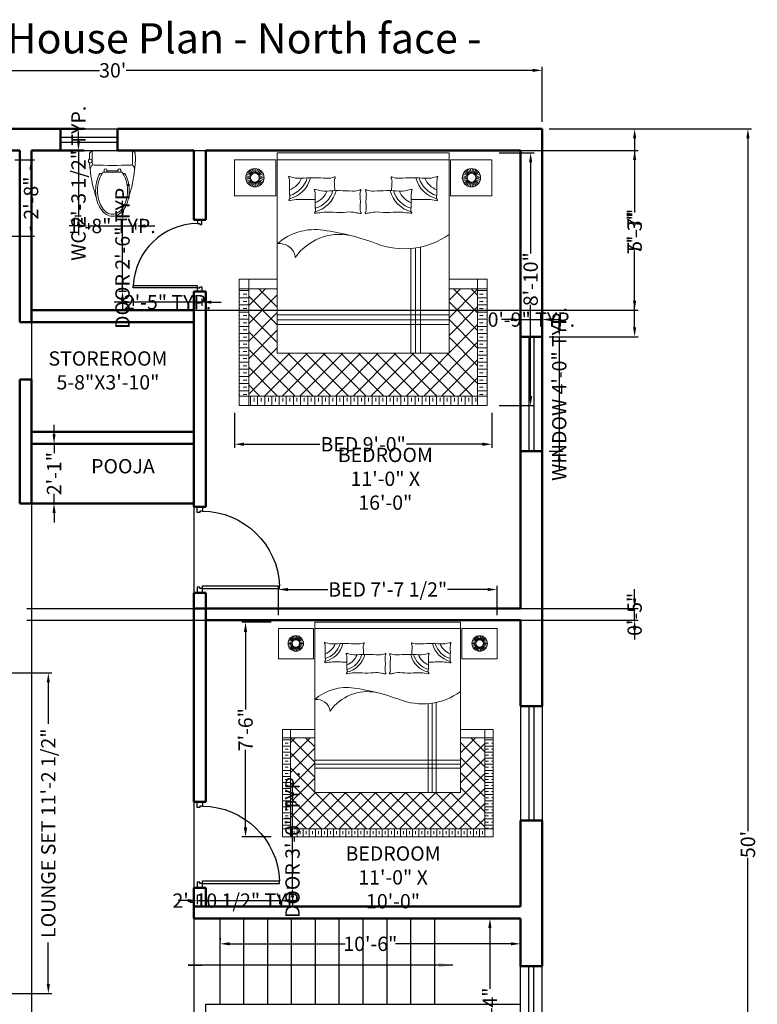
# Model space of a CAD drawing. Units: inches. Extents: x 234 to 707, y 260 to 1025.
# Tile 3 of 3: x 398 to 707, y 612 to 1025. Entities that reach past the tile are written whole.
import ezdxf

# ---------------------------------------------------------------- set-up
doc = ezdxf.new("R2010")
doc.units = ezdxf.units.IN
doc.header["$MEASUREMENT"] = 0
for name, color, linetype, lineweight in [('A-ANNO-DIMS', 3, 'Continuous', 18), ('A-ANNO-SYMB', 3, 'Continuous', 18), ('A-ANNO-TEXT', 7, 'Continuous', 35), ('A-AREA-IDEN', 7, 'Continuous', 25), ('A-DOOR', 2, 'Continuous', 25), ('A-FLOR-CASE', 30, 'Continuous', 25), ('A-FLOR-FIXT', 9, 'Continuous', 18), ('A-FLOR-STRS', 4, 'Continuous', 25), ('A-FURN', 9, 'Continuous', 18), ('WALL', 7, 'Continuous', 50), ('WINDOW', 2, 'Continuous', 25)]:
    doc.layers.add(name, color=color, linetype=linetype, lineweight=lineweight)
doc.styles.get("Standard").update_dxf_attribs({"font": 'arial.ttf'})
doc.styles.add('YQ_DIM', font='SUPEROS.SHX', dxfattribs={"width": 0.8, "bigfont": 'HZDX.SHX'})
doc.dimstyles.new('yqi0', dxfattribs={"dimscale": 0, "dimtxt": 6, "dimasz": 4, "dimexe": 1.5, "dimexo": 3, "dimgap": 0.5, "dimtad": 0, "dimdec": 1, "dimdsep": 46, "dimlunit": 4, "dimtxsty": 'Standard', "dimcen": 0, "dimclrd": 256, "dimclre": 256, "dimclrt": 7, "dimadec": 1, "dimazin": 2, "dimtfac": 1, "dimtdec": 1, "dimtix": 1, "dimtmove": 2, "dimatfit": 2, "dimfxl": 1, "dimtolj": 1, "dimtzin": 0, "dimarcsym": 0})

# ---------------------------------------------------------------- blocks, each defined once
blk = doc.blocks.new('*D2')
at = {"layer": 'A-ANNO-DIMS', "color": 0, "lineweight": -2, "transparency": 16777216}
for p, q in [((257.21, 981.74), (257.21, 1004.79)), ((261.21, 1003.29), (431.62, 1003.29)), ((613.21, 1003.29), (442.8, 1003.29)), ((617.21, 981.74), (617.21, 1004.79))]:
    blk.add_line(p, q, dxfattribs=at)
at = {"layer": 'A-ANNO-DIMS', "color": 0, "transparency": 16777216}
for points in [[(261.21, 1003.95), (261.21, 1002.62), (257.21, 1003.29)], [(613.21, 1003.95), (613.21, 1002.62), (617.21, 1003.29)]]:
    blk.add_solid(points, dxfattribs=at)
at = {"layer": 'Defpoints', "color": 0, "transparency": 16777216}
for p in [(617.21, 1003.29), (257.21, 978.74), (617.21, 978.74)]:
    blk.add_point(p, dxfattribs=at)
at = {"layer": 'A-ANNO-DIMS', "color": 0, "transparency": 16777216, "insert": (437.21, 1003.29), "char_height": 6, "attachment_point": 5}
blk.add_mtext("\\A1;30'", dxfattribs=at)
blk = doc.blocks.new('*D3')
at = {"layer": 'A-ANNO-DIMS', "color": 0, "lineweight": -2, "transparency": 16777216}
for p, q in [((620.21, 978.74), (705.01, 978.74)), ((703.51, 974.74), (703.51, 684.33)), ((703.51, 382.74), (703.51, 673.15)), ((620.21, 378.74), (705.01, 378.74))]:
    blk.add_line(p, q, dxfattribs=at)
at = {"layer": 'A-ANNO-DIMS', "color": 0, "transparency": 16777216}
for points in [[(702.84, 974.74), (704.17, 974.74), (703.51, 978.74)], [(702.84, 382.74), (704.17, 382.74), (703.51, 378.74)]]:
    blk.add_solid(points, dxfattribs=at)
at = {"layer": 'Defpoints', "color": 0, "transparency": 16777216}
for p in [(617.21, 978.74), (617.21, 378.74), (703.51, 378.74)]:
    blk.add_point(p, dxfattribs=at)
at = {"layer": 'A-ANNO-DIMS', "color": 0, "transparency": 16777216, "insert": (703.51, 678.74), "char_height": 6, "attachment_point": 5, "rotation": 90}
blk.add_mtext("\\A1;50'", dxfattribs=at)
blk = doc.blocks.new('DR_D01')
for p, q in [((-0.45, 0.93), (-0.42, 0.93)), ((-0.45, 0.03), (-0.45, 0.93)), ((-0.42, 0.03), (-0.42, 0.93)), ((-0.5, 0.03), (-0.42, 0.03)), ((-0.5, 0.03), (-0.5, -0.03)), ((-0.45, 0.03), (-0.45, 0)), ((-0.45, 0), (-0.435, 0)), ((-0.435, 0), (-0.435, -0.03)), ((0.435, 0), (0.435, -0.03)), ((0.45, 0), (0.435, 0)), ((0.45, 0.03), (0.45, 0)), ((0.5, 0.03), (0.45, 0.03)), ((0.5, -0.03), (0.5, 0.03)), ((-0.435, -0.03), (-0.5, -0.03)), ((0.435, -0.03), (0.5, -0.03))]:
    blk.add_line(p, q)
blk.add_arc((-0.46, 0.021), 0.91, 0.5915, 87.4664)
blk = doc.blocks.new('WD_WIN4')
for p, q in [((-0.5, 0.5), (0.5, 0.5)), ((-0.5, 0.12), (0.5, 0.12)), ((-0.5, -0.12), (0.5, -0.12)), ((-0.5, -0.5), (0.5, -0.5))]:
    blk.add_line(p, q)
blk = doc.blocks.new('yq_matong_01')
for p, q in [((20, 221), (139, 221)), ((0, 201), (0, -201)), ((252, 138), (252, 114)), ((216, 91), (238, 91)), ((216, 61), (238, 61)), ((223, 61), (223, -61)), ((238, 104), (238, -104)), ((216, -61), (238, -61)), ((216, -91), (238, -91)), ((252, -114), (252, -138)), ((20, -221), (139, -221)), ((97, -221), (97, -226)), ((97, -226), (132, -226)), ((132, -221), (132, -226))]:
    blk.add_line(p, q)
for centre, radius, start, end in [((55, 202), 54.8, 117.322, 181.8992), ((20, 201), 20, 90, 180), ((64, -1165), 1417, 71.4068, 91.3856), ((139, 201), 20, 2.3063, 90), ((217, 161), 83.2, 95.4963, 139.9324), ((-4840, 0), 5003, 357.6937, 2.3063), ((357, -47), 193, 123.2779, 128.1384), ((407, -123), 283, 105.2088, 123.2779), ((407, -123), 303, 105.2088, 120.5699), ((439, -242), 427, 74.7912, 105.2088), ((439, -242), 407, 74.7912, 105.2088), ((471, -123), 283, 56.7221, 74.7912), ((471, -123), 303, 56.7221, 74.7912), ((521, -47), 193, 32.2565, 56.7221), ((521, -47), 213, 32.2565, 56.7221), ((216, 76), 15, 90, 270), ((596, 0), 104, 360, 32.2565), ((596, 0), 124, 360, 32.2565), ((216, -76), 15, 90, 270), ((357, 47), 193, 231.8616, 236.7221), ((521, 47), 193, 303.2779, 327.7435), ((521, 47), 213, 303.2779, 327.7435), ((596, 0), 104, 327.7435, 360), ((596, 0), 124, 327.7435, 360), ((51, -204), 51.4, 175.687, 245.0918), ((20, -201), 20, 180, 270), ((64, 1165), 1417, 272.8967, 288.5932), ((139, -201), 20, 270, 357.6937), ((217, -161), 83.2, 220.0676, 264.5037), ((407, 123), 283, 236.7221, 254.7912), ((407, 123), 303, 239.4301, 254.7912), ((439, 242), 427, 254.7912, 285.2088), ((439, 242), 407, 254.7912, 285.2088), ((471, 123), 283, 285.2088, 303.2779), ((471, 123), 303, 285.2088, 303.2779), ((64, 1165), 1417, 268.6144, 271.2036), ((157, -247), 63.1, 159.6834, 188.4939), ((114, -226), 37, 237.5287, 304.2772), ((72, -247), 63.1, 352.0944, 20.3166)]:
    blk.add_arc(centre, radius, start, end)
blk = doc.blocks.new('BED')
h = blk.add_hatch()
h.set_pattern_fill('TRANS', color=256, scale=12, style=0)
h.set_pattern_definition([(360, (4433.967, -9715.0492), (1e-15, 3), []), (360, (4433.967, -9713.5492), (1e-15, 3), [1.5, -1.5])])
h.paths.add_polyline_path([(48, -103), (52, -103), (52, -58), (48, -58)])
h.paths.add_polyline_path([(-48, -58), (-52, -58), (-52, -103), (-48, -103)])
h = blk.add_hatch()
h.set_pattern_fill('ANSI37', color=256, scale=42, angle=-90, style=0)
h.set_pattern_definition([(315, (7787.1367, 4477.8466), (3.7123106, 3.7123106), []), (45, (7787.1367, 4477.8466), (-3.7123106, 3.7123106), [])])
h.paths.add_polyline_path([(-36, -85), (-36, -58), (-48, -58), (-48, -103), (48, -103), (48, -58), (36, -58), (36, -85)])
h = blk.add_hatch()
h.set_pattern_fill('TRANS', color=256, scale=12, angle=-90, style=0)
h.set_pattern_definition([(270, (4433.967, -9715.0492), (3, -1e-15), []), (270, (4435.467, -9715.0492), (3, -1e-15), [1.5, -1.5])])
h.paths.add_polyline_path([(48, -107), (48, -103), (-48, -103), (-48, -107)])
for p, q in [((-54, -4), (-54, -19)), ((-36.64, -4), (-54, -4)), ((-36.64, -4), (-36.64, -19)), ((-36, -1), (36, -1)), ((-36, -85), (-36, -1)), ((-36, -4), (36, -4)), ((36, -1), (36, -85)), ((36.64, -4), (36.64, -19)), ((36.64, -4), (54, -4)), ((54, -4), (54, -19)), ((-46.31, -9.86), (-47.31, -8.13)), ((-45.96, -9.7), (-46.58, -7.8)), ((-45.58, -9.62), (-45.8, -7.63)), ((-45.2, -9.62), (-45, -7.63)), ((-44.82, -9.7), (-44.21, -7.79)), ((-44.47, -9.85), (-43.48, -8.12)), ((44.47, -9.85), (43.48, -8.12)), ((44.82, -9.7), (44.21, -7.79)), ((45.2, -9.62), (45, -7.63)), ((45.58, -9.62), (45.8, -7.63)), ((45.96, -9.7), (46.58, -7.8)), ((46.31, -9.86), (47.31, -8.13)), ((-47.23, -11.45), (-49.23, -11.45)), ((-47.19, -11.07), (-49.14, -10.66)), ((-47.19, -11.83), (-49.14, -12.25)), ((-47.07, -10.7), (-48.9, -9.89)), ((-47.07, -12.2), (-48.89, -13.01)), ((-46.88, -10.37), (-48.5, -9.2)), ((-46.62, -10.08), (-47.96, -8.6)), ((-44.16, -10.08), (-42.83, -8.59)), ((-43.9, -10.36), (-42.29, -9.18)), ((-43.71, -10.7), (-41.89, -9.88)), ((-43.71, -12.19), (-41.88, -13)), ((-43.59, -11.06), (-41.64, -10.64)), ((-43.59, -11.83), (-41.63, -12.24)), ((-43.55, -11.44), (-41.55, -11.44)), ((43.55, -11.44), (41.55, -11.44)), ((43.59, -11.83), (41.63, -12.24)), ((43.59, -11.06), (41.64, -10.64)), ((43.71, -12.19), (41.88, -13)), ((43.71, -10.7), (41.89, -9.88)), ((43.9, -10.36), (42.29, -9.18)), ((44.16, -10.08), (42.83, -8.59)), ((46.62, -10.08), (47.96, -8.6)), ((46.88, -10.37), (48.5, -9.2)), ((47.07, -10.7), (48.9, -9.89)), ((47.07, -12.2), (48.89, -13.01)), ((47.19, -11.07), (49.14, -10.66)), ((47.19, -11.83), (49.14, -12.25)), ((47.23, -11.45), (49.23, -11.45)), ((-46.87, -12.53), (-48.49, -13.71)), ((-46.62, -12.81), (-47.95, -14.3)), ((-46.3, -13.04), (-47.3, -14.77)), ((-45.95, -13.2), (-46.57, -15.1)), ((-45.58, -13.27), (-45.78, -15.26)), ((-45.19, -13.27), (-44.98, -15.26)), ((-44.82, -13.19), (-44.2, -15.09)), ((-44.47, -13.04), (-43.46, -14.77)), ((-44.16, -12.81), (-42.82, -14.29)), ((-43.9, -12.52), (-42.28, -13.7)), ((43.9, -12.52), (42.28, -13.7)), ((44.16, -12.81), (42.82, -14.29)), ((44.47, -13.04), (43.46, -14.77)), ((44.82, -13.19), (44.2, -15.09)), ((45.19, -13.27), (44.98, -15.26)), ((45.58, -13.27), (45.78, -15.26)), ((45.95, -13.2), (46.57, -15.1)), ((46.3, -13.04), (47.3, -14.77)), ((46.62, -12.81), (47.95, -14.3)), ((46.87, -12.53), (48.49, -13.71)), ((-36.64, -19), (-54, -19)), ((36.64, -19), (54, -19)), ((20, -85), (20, -41.14)), ((22, -85), (22, -40.91)), ((24, -85), (24, -40.55)), ((-52, -54), (-52, -107)), ((-52, -54), (-36, -54)), ((-48, -54), (-48, -107)), ((36, -54), (52, -54)), ((48, -54), (48, -107)), ((52, -54), (52, -107)), ((-52, -58), (-36, -58)), ((36, -58), (52, -58)), ((36, -69), (-36, -69)), ((36, -71), (-36, -71)), ((36, -73), (-36, -73)), ((36, -85), (-36, -85)), ((-52, -103), (52, -103)), ((-52, -107), (52, -107))]:
    blk.add_line(p, q)
for centre, radius in [((-45.39, -11.45), 3.84), ((45.39, -11.45), 3.84), ((-45.39, -11.45), 1.84), ((45.39, -11.45), 1.84)]:
    blk.add_circle(centre, radius)
for centre, radius, start, end in [((-30.92, -11.24), 0.328, 35.8976, 208.6272), ((-42.38, -17.5), 12.73, 27.1629, 28.6272), ((-44.37, -13.89), 13.5, 357.4804, 9.3956), ((-33.8, -8.61), 8.46, 289.8695, 338.9843), ((-33.8, -8.61), 12.06, 283.8498, 346.0842), ((-33.8, -8.61), 10.71, 286.0319, 344.1205), ((-26.84, 0.13), 11.82, 251.1782, 273.3982), ((-20.92, -99.64), 88.13, 86.2964, 93.3982), ((-14.79, -4.98), 6.73, 266.2964, 294.303), ((-8.24, -13.16), 3.86, 159.0146, 186.273), ((-11.92, -11.33), 0.242, 335.7259, 114.303), ((-5.69, -14.14), 6.59, 155.7259, 159.0146), ((11.92, -11.33), 0.242, 65.697, 204.2741), ((5.69, -14.14), 6.59, 20.9854, 24.2741), ((8.24, -13.16), 3.86, 353.727, 20.9854), ((14.79, -4.98), 6.73, 245.697, 273.7036), ((20.92, -99.64), 88.13, 86.6018, 93.7036), ((33.8, -8.61), 12.06, 193.9158, 256.1502), ((33.8, -8.61), 10.71, 195.8795, 253.9681), ((33.8, -8.61), 8.46, 201.0157, 250.1305), ((26.84, 0.13), 11.82, 266.6018, 288.8218), ((30.92, -11.24), 0.328, 331.3728, 144.1024), ((44.37, -13.89), 13.5, 170.6044, 182.5196), ((42.38, -17.5), 12.73, 151.3728, 152.8371), ((10.15, -16.29), 41.07, 177.4804, 184.5075), ((-20.16, -16.62), 0.328, 35.8976, 208.6272), ((-16.08, -5.24), 11.82, 251.1782, 273.3982), ((-36.64, -16.28), 24.71, 358.5721, 6.273), ((-4.03, -10.35), 6.73, 266.2964, 294.303), ((-1.16, -16.7), 0.242, 335.7259, 114.303), ((1.16, -16.7), 0.242, 65.697, 204.2741), ((4.03, -10.35), 6.73, 245.697, 273.7036), ((36.64, -16.28), 24.71, 173.727, 181.4279), ((16.08, -5.24), 11.82, 266.6018, 288.8218), ((20.16, -16.62), 0.328, 331.3728, 144.1024), ((-10.15, -16.29), 41.07, 355.4925, 2.5196), ((-32.72, -19.65), 1.93, 327.6219, 339.2246), ((-32.67, -19.67), 1.88, 339.2246, 4.5075), ((-25.16, -53.53), 33, 93.5164, 99.6766), ((-25.27, -51.86), 31.33, 86.4836, 93.5164), ((-21.12, 15.68), 36.34, 266.4836, 271.5234), ((-31.62, -22.87), 12.73, 27.1629, 28.6272), ((-33.61, -19.26), 13.5, 357.4804, 9.3956), ((-23.04, -13.99), 8.46, 289.8695, 338.9843), ((20.91, -21.66), 41.07, 177.4804, 184.5075), ((-23.04, -13.99), 12.06, 283.8498, 346.0842), ((-23.04, -13.99), 10.71, 286.0319, 344.1205), ((-10.15, -105.01), 88.13, 86.2964, 93.3982), ((2.52, -18.53), 3.86, 159.0146, 186.273), ((-25.88, -21.66), 24.71, 354.3784, 6.273), ((5.07, -19.51), 6.59, 155.7259, 159.0146), ((-5.07, -19.51), 6.59, 20.9854, 24.2741), ((-2.52, -18.53), 3.86, 353.727, 20.9854), ((25.88, -21.66), 24.71, 173.727, 185.6216), ((10.15, -105.01), 88.13, 86.6018, 93.7036), ((23.04, -13.99), 12.06, 193.9158, 256.1502), ((23.04, -13.99), 10.71, 195.8795, 253.9681), ((23.04, -13.99), 8.46, 201.0157, 250.1305), ((-20.91, -21.66), 41.07, 355.4925, 2.5196), ((33.61, -19.26), 13.5, 170.6044, 182.5196), ((21.12, 15.68), 36.34, 268.4766, 273.5164), ((31.62, -22.87), 12.73, 151.3728, 152.8371), ((25.27, -51.86), 31.33, 86.4836, 93.5164), ((25.16, -53.53), 33, 80.3234, 86.4836), ((32.67, -19.67), 1.88, 175.4925, 200.7754), ((32.72, -19.65), 1.93, 200.7754, 212.3781), ((-30.88, -20.82), 0.25, 147.6219, 311.9343), ((2.55, -24.46), 3.86, 174.3784, 204.7617), ((-2.55, -24.46), 3.86, 335.2383, 5.6216), ((30.88, -20.82), 0.25, 228.0657, 32.3781), ((-20.12, -26.19), 0.25, 147.6219, 311.9343), ((-21.96, -25.02), 1.93, 327.6219, 339.2246), ((-21.91, -25.04), 1.88, 339.2246, 4.5075), ((-14.4, -58.9), 33, 93.5164, 99.6766), ((-14.51, -57.23), 31.33, 86.4836, 93.5164), ((-10.35, 10.3), 36.34, 266.4836, 275.306), ((-5.78, -38.98), 13.15, 77.9645, 95.306), ((2.5, -0.17), 26.53, 257.9645, 261.9243), ((-1.09, -26.25), 0.228, 231.9005, 52.8902), ((1.09, -26.25), 0.228, 127.1098, 308.0995), ((-2.5, -0.17), 26.53, 278.0757, 282.0355), ((5.78, -38.98), 13.15, 84.694, 102.0355), ((10.35, 10.3), 36.34, 264.694, 273.5164), ((14.51, -57.23), 31.33, 86.4836, 93.5164), ((14.4, -58.9), 33, 80.3234, 86.4836), ((20.12, -26.19), 0.25, 228.0657, 32.3781), ((21.91, -25.04), 1.88, 175.4925, 200.7754), ((21.96, -25.02), 1.93, 200.7754, 212.3781), ((-20.27, -56.85), 23.66, 81.0857, 131.6581), ((-9.91, -57.83), 22.61, 78.6456, 145.1521), ((-32.56, -143.87), 111.55, 70.0977, 81.7735), ((17.27, -9.21), 32.05, 248.2778, 305.7663), ((-34.97, -45.63), 6.55, 6.3172, 99.0807)]:
    blk.add_arc(centre, radius, start, end)
blk = doc.blocks.new('*D14')
at = {"layer": 'A-ANNO-DIMS', "color": 0, "lineweight": -2, "transparency": 16777216}
for p, q in [((482.21, 639.45), (482.21, 638.6)), ((486.21, 637.1), (534.69, 637.1)), ((604.21, 637.1), (555.74, 637.1)), ((608.21, 639.45), (608.21, 638.6))]:
    blk.add_line(p, q, dxfattribs=at)
at = {"layer": 'A-ANNO-DIMS', "color": 0, "transparency": 16777216}
for points in [[(486.21, 637.77), (486.21, 636.44), (482.21, 637.1)], [(604.21, 637.77), (604.21, 636.44), (608.21, 637.1)]]:
    blk.add_solid(points, dxfattribs=at)
at = {"layer": 'Defpoints', "color": 0, "transparency": 16777216}
for p in [(482.21, 636.45), (608.21, 637.1), (608.21, 636.45)]:
    blk.add_point(p, dxfattribs=at)
at = {"layer": 'A-ANNO-DIMS', "color": 0, "transparency": 16777216, "insert": (545.21, 637.1), "char_height": 6, "attachment_point": 5}
blk.add_mtext('\\A1;10\'-6"', dxfattribs=at)
blk = doc.blocks.new('*D16')
at = {"layer": 'A-ANNO-DIMS', "color": 0, "lineweight": -2, "transparency": 16777216}
for p, q in [((598, 647.74), (596.84, 647.74)), ((595.34, 643.74), (595.34, 618.23)), ((595.34, 575.74), (595.34, 601.25)), ((598, 571.74), (596.84, 571.74))]:
    blk.add_line(p, q, dxfattribs=at)
at = {"layer": 'A-ANNO-DIMS', "color": 0, "transparency": 16777216}
for points in [[(594.67, 643.74), (596, 643.74), (595.34, 647.74)], [(594.67, 575.74), (596, 575.74), (595.34, 571.74)]]:
    blk.add_solid(points, dxfattribs=at)
at = {"layer": 'Defpoints', "color": 0, "transparency": 16777216}
for p in [(595, 647.74), (595.34, 647.74), (595, 571.74)]:
    blk.add_point(p, dxfattribs=at)
at = {"layer": 'A-ANNO-DIMS', "color": 0, "transparency": 16777216, "insert": (595.34, 609.74), "char_height": 6, "attachment_point": 5, "rotation": 90}
blk.add_mtext('\\A1;6\'-4"', dxfattribs=at)
blk = doc.blocks.new('*D17')
at = {"layer": 'A-ANNO-DIMS', "color": 0, "lineweight": -2, "transparency": 16777216}
for p, q in [((412.62, 850.74), (412.62, 854.74)), ((412.39, 846.74), (414.12, 846.74)), ((412.62, 846.74), (412.62, 842.77)), ((412.62, 821.74), (412.62, 825.72)), ((412.39, 821.74), (414.12, 821.74)), ((412.62, 817.74), (412.62, 813.74))]:
    blk.add_line(p, q, dxfattribs=at)
at = {"layer": 'A-ANNO-DIMS', "color": 0, "transparency": 16777216}
for points in [[(411.96, 850.74), (413.29, 850.74), (412.62, 846.74)], [(411.96, 817.74), (413.29, 817.74), (412.62, 821.74)]]:
    blk.add_solid(points, dxfattribs=at)
at = {"layer": 'Defpoints', "color": 0, "transparency": 16777216}
for p in [(409.39, 846.74), (409.39, 821.74), (412.62, 821.74)]:
    blk.add_point(p, dxfattribs=at)
at = {"layer": 'A-ANNO-DIMS', "color": 0, "transparency": 16777216, "insert": (412.62, 834.24), "char_height": 6, "attachment_point": 5, "rotation": 90}
blk.add_mtext('\\A1;2\'-1"', dxfattribs=at)
blk = doc.blocks.new('*D21')
at = {"layer": 'A-ANNO-DIMS', "lineweight": -2, "transparency": 16777216}
for p, q in [((624.41, 895.61), (624.41, 899.61)), ((620.21, 891.61), (625.91, 891.61)), ((624.41, 891.61), (624.41, 843.61)), ((620.21, 843.61), (625.91, 843.61)), ((624.41, 839.61), (624.41, 835.61))]:
    blk.add_line(p, q, dxfattribs=at)
at = {"layer": 'A-ANNO-DIMS', "transparency": 16777216}
for points in [[(623.75, 895.61), (625.08, 895.61), (624.41, 891.61)], [(623.75, 839.61), (625.08, 839.61), (624.41, 843.61)]]:
    blk.add_solid(points, dxfattribs=at)
at = {"layer": 'Defpoints', "color": 0, "transparency": 16777216}
for p in [(617.21, 891.61), (617.21, 843.61), (624.41, 843.61)]:
    blk.add_point(p, dxfattribs=at)
at = {"layer": 'A-ANNO-DIMS', "color": 7, "transparency": 16777216, "insert": (624.41, 867.61), "char_height": 6, "attachment_point": 5, "rotation": 90}
blk.add_mtext('\\A1;WINDOW 4\'-0" TYP.', dxfattribs=at)
blk = doc.blocks.new('*D22')
at = {"layer": 'A-ANNO-DIMS', "lineweight": -2, "transparency": 16777216}
for p, q in [((608.21, 894.61), (608.21, 900.31)), ((617.21, 894.61), (617.21, 900.31)), ((604.21, 898.81), (600.21, 898.81)), ((608.21, 898.81), (617.21, 898.81)), ((621.21, 898.81), (625.21, 898.81))]:
    blk.add_line(p, q, dxfattribs=at)
at = {"layer": 'A-ANNO-DIMS', "transparency": 16777216}
for points in [[(604.21, 899.48), (604.21, 898.15), (608.21, 898.81)], [(621.21, 899.48), (621.21, 898.15), (617.21, 898.81)]]:
    blk.add_solid(points, dxfattribs=at)
at = {"layer": 'Defpoints', "color": 0, "transparency": 16777216}
for p in [(617.21, 898.81), (608.21, 891.61), (617.21, 891.61)]:
    blk.add_point(p, dxfattribs=at)
at = {"layer": 'A-ANNO-DIMS', "color": 7, "transparency": 16777216, "insert": (612.71, 898.81), "char_height": 6, "attachment_point": 5}
blk.add_mtext('\\A1;0\'-9" TYP.', dxfattribs=at)
blk = doc.blocks.new('*D27')
at = {"layer": 'A-ANNO-DIMS', "lineweight": -2, "transparency": 16777216}
for p, q in [((512.59, 700.62), (512.59, 704.62)), ((510.19, 696.62), (514.09, 696.62)), ((512.59, 660.62), (512.59, 696.62)), ((510.19, 660.62), (514.09, 660.62)), ((512.59, 656.62), (512.59, 652.62))]:
    blk.add_line(p, q, dxfattribs=at)
at = {"layer": 'A-ANNO-DIMS', "transparency": 16777216}
for points in [[(511.93, 700.62), (513.26, 700.62), (512.59, 696.62)], [(511.93, 656.62), (513.26, 656.62), (512.59, 660.62)]]:
    blk.add_solid(points, dxfattribs=at)
at = {"layer": 'Defpoints', "color": 0, "transparency": 16777216}
for p in [(507.19, 696.62), (512.59, 696.62), (507.19, 660.62)]:
    blk.add_point(p, dxfattribs=at)
at = {"layer": 'A-ANNO-DIMS', "color": 7, "transparency": 16777216, "insert": (512.59, 678.62), "char_height": 6, "attachment_point": 5, "rotation": 90}
blk.add_mtext('\\A1;DOOR 3\'-0" TYP.', dxfattribs=at)
blk = doc.blocks.new('*D28')
at = {"layer": 'A-ANNO-DIMS', "lineweight": -2, "transparency": 16777216}
for p, q in [((472.63, 657.62), (472.63, 653.72)), ((507.19, 657.62), (507.19, 653.72)), ((468.63, 655.22), (464.63, 655.22)), ((472.63, 655.22), (507.19, 655.22)), ((511.19, 655.22), (515.19, 655.22))]:
    blk.add_line(p, q, dxfattribs=at)
at = {"layer": 'A-ANNO-DIMS', "transparency": 16777216}
for points in [[(468.63, 655.88), (468.63, 654.55), (472.63, 655.22)], [(511.19, 655.88), (511.19, 654.55), (507.19, 655.22)]]:
    blk.add_solid(points, dxfattribs=at)
at = {"layer": 'Defpoints', "color": 0, "transparency": 16777216}
for p in [(472.63, 660.62), (507.19, 660.62), (507.19, 655.22)]:
    blk.add_point(p, dxfattribs=at)
at = {"layer": 'A-ANNO-DIMS', "color": 7, "transparency": 16777216, "insert": (489.91, 655.22), "char_height": 6, "attachment_point": 5}
blk.add_mtext('\\A1;2\'-10 1/2" TYP.', dxfattribs=at)
blk = doc.blocks.new('*D29')
at = {"layer": 'A-ANNO-DIMS', "lineweight": -2, "transparency": 16777216}
for p, q in [((441.31, 944.62), (441.31, 948.62)), ((442.81, 940.62), (439.81, 940.62)), ((441.31, 910.62), (441.31, 940.62)), ((442.81, 910.62), (439.81, 910.62)), ((441.31, 906.62), (441.31, 902.62))]:
    blk.add_line(p, q, dxfattribs=at)
at = {"layer": 'A-ANNO-DIMS', "transparency": 16777216}
for points in [[(440.65, 944.62), (441.98, 944.62), (441.31, 940.62)], [(440.65, 906.62), (441.98, 906.62), (441.31, 910.62)]]:
    blk.add_solid(points, dxfattribs=at)
at = {"layer": 'Defpoints', "color": 0, "transparency": 16777216}
for p in [(441.31, 940.62), (445.81, 940.62), (445.81, 910.62)]:
    blk.add_point(p, dxfattribs=at)
at = {"layer": 'A-ANNO-DIMS', "color": 7, "transparency": 16777216, "insert": (441.31, 925.62), "char_height": 6, "attachment_point": 5, "rotation": 90}
blk.add_mtext('\\A1;DOOR 2\'-6" TYP.', dxfattribs=at)
blk = doc.blocks.new('*D30')
at = {"layer": 'A-ANNO-DIMS', "lineweight": -2, "transparency": 16777216}
for p, q in [((441.81, 906.12), (437.81, 906.12)), ((445.81, 907.62), (445.81, 904.62)), ((474.61, 906.12), (445.81, 906.12)), ((474.61, 907.62), (474.61, 904.62)), ((478.61, 906.12), (482.61, 906.12))]:
    blk.add_line(p, q, dxfattribs=at)
at = {"layer": 'A-ANNO-DIMS', "transparency": 16777216}
for points in [[(441.81, 906.78), (441.81, 905.45), (445.81, 906.12)], [(478.61, 906.78), (478.61, 905.45), (474.61, 906.12)]]:
    blk.add_solid(points, dxfattribs=at)
at = {"layer": 'Defpoints', "color": 0, "transparency": 16777216}
for p in [(445.81, 910.62), (474.61, 910.62), (445.81, 906.12)]:
    blk.add_point(p, dxfattribs=at)
at = {"layer": 'A-ANNO-DIMS', "color": 7, "transparency": 16777216, "insert": (460.21, 906.12), "char_height": 6, "attachment_point": 5}
blk.add_mtext('\\A1;2\'-5" TYP.', dxfattribs=at)
blk = doc.blocks.new('*D31')
at = {"layer": 'A-ANNO-DIMS', "lineweight": -2, "transparency": 16777216}
for p, q in [((488.21, 859.74), (488.21, 845.04)), ((596.21, 859.74), (596.21, 845.04)), ((492.21, 846.54), (524.09, 846.54)), ((592.21, 846.54), (560.34, 846.54))]:
    blk.add_line(p, q, dxfattribs=at)
at = {"layer": 'A-ANNO-DIMS', "transparency": 16777216}
for points in [[(492.21, 847.21), (492.21, 845.87), (488.21, 846.54)], [(592.21, 847.21), (592.21, 845.87), (596.21, 846.54)]]:
    blk.add_solid(points, dxfattribs=at)
at = {"layer": 'Defpoints', "color": 0, "transparency": 16777216}
for p in [(488.21, 862.74), (596.21, 862.74), (596.21, 846.54)]:
    blk.add_point(p, dxfattribs=at)
at = {"layer": 'A-ANNO-DIMS', "color": 7, "transparency": 16777216, "insert": (542.21, 846.54), "char_height": 6, "attachment_point": 5}
blk.add_mtext('\\A1;BED 9\'-0"', dxfattribs=at)
blk = doc.blocks.new('*D32')
at = {"layer": 'A-ANNO-DIMS', "lineweight": -2, "transparency": 16777216}
for p, q in [((599.21, 968.74), (613.91, 968.74)), ((612.41, 964.74), (612.41, 926.55)), ((612.41, 866.74), (612.41, 904.93)), ((599.21, 862.74), (613.91, 862.74))]:
    blk.add_line(p, q, dxfattribs=at)
at = {"layer": 'A-ANNO-DIMS', "transparency": 16777216}
for points in [[(611.75, 964.74), (613.08, 964.74), (612.41, 968.74)], [(611.75, 866.74), (613.08, 866.74), (612.41, 862.74)]]:
    blk.add_solid(points, dxfattribs=at)
at = {"layer": 'Defpoints', "color": 0, "transparency": 16777216}
for p in [(596.21, 968.74), (612.41, 968.74), (596.21, 862.74)]:
    blk.add_point(p, dxfattribs=at)
at = {"layer": 'A-ANNO-DIMS', "color": 7, "transparency": 16777216, "insert": (612.41, 915.74), "char_height": 6, "attachment_point": 5, "rotation": 90}
blk.add_mtext('\\A1;8\'-10"', dxfattribs=at)
blk = doc.blocks.new('*D33')
at = {"layer": 'A-ANNO-DIMS', "lineweight": -2, "transparency": 16777216}
for p, q in [((506.65, 774.89), (506.65, 787.15)), ((510.65, 785.65), (527.38, 785.65)), ((594.35, 785.65), (577.61, 785.65)), ((598.35, 774.89), (598.35, 787.15))]:
    blk.add_line(p, q, dxfattribs=at)
at = {"layer": 'A-ANNO-DIMS', "transparency": 16777216}
for points in [[(510.65, 786.31), (510.65, 784.98), (506.65, 785.65)], [(594.35, 786.31), (594.35, 784.98), (598.35, 785.65)]]:
    blk.add_solid(points, dxfattribs=at)
at = {"layer": 'Defpoints', "color": 0, "transparency": 16777216}
for p in [(598.35, 785.65), (506.65, 771.89), (598.35, 771.89)]:
    blk.add_point(p, dxfattribs=at)
at = {"layer": 'A-ANNO-DIMS', "color": 7, "transparency": 16777216, "insert": (552.5, 785.65), "char_height": 6, "attachment_point": 5}
blk.add_mtext('\\A1;BED 7\'-7 1/2"', dxfattribs=at)
blk = doc.blocks.new('*D34')
at = {"layer": 'A-ANNO-DIMS', "lineweight": -2, "transparency": 16777216}
for p, q in [((503.65, 771.89), (491.39, 771.89)), ((492.89, 767.89), (492.89, 735.34)), ((492.89, 685.89), (492.89, 718.44)), ((503.65, 681.89), (491.39, 681.89))]:
    blk.add_line(p, q, dxfattribs=at)
at = {"layer": 'A-ANNO-DIMS', "transparency": 16777216}
for points in [[(492.22, 767.89), (493.56, 767.89), (492.89, 771.89)], [(492.22, 685.89), (493.56, 685.89), (492.89, 681.89)]]:
    blk.add_solid(points, dxfattribs=at)
at = {"layer": 'Defpoints', "color": 0, "transparency": 16777216}
for p in [(492.89, 771.89), (506.65, 771.89), (506.65, 681.89)]:
    blk.add_point(p, dxfattribs=at)
at = {"layer": 'A-ANNO-DIMS', "color": 7, "transparency": 16777216, "insert": (492.89, 726.89), "char_height": 6, "attachment_point": 5, "rotation": 90}
blk.add_mtext('\\A1;7\'-6"', dxfattribs=at)
blk = doc.blocks.new('*D37')
at = {"layer": 'A-ANNO-DIMS', "lineweight": -2, "transparency": 16777216}
for p, q in [((422.86, 973.72), (422.86, 977.72)), ((423.99, 969.72), (421.36, 969.72)), ((422.86, 969.72), (422.86, 942.18)), ((423.99, 942.18), (421.36, 942.18)), ((422.86, 938.18), (422.86, 934.18))]:
    blk.add_line(p, q, dxfattribs=at)
at = {"layer": 'A-ANNO-DIMS', "transparency": 16777216}
for points in [[(422.19, 973.72), (423.53, 973.72), (422.86, 969.72)], [(422.19, 938.18), (423.53, 938.18), (422.86, 942.18)]]:
    blk.add_solid(points, dxfattribs=at)
at = {"layer": 'Defpoints', "color": 0, "transparency": 16777216}
for p in [(426.99, 969.72), (422.86, 942.18), (426.99, 942.18)]:
    blk.add_point(p, dxfattribs=at)
at = {"layer": 'A-ANNO-DIMS', "color": 7, "transparency": 16777216, "insert": (422.86, 955.95), "char_height": 6, "attachment_point": 5, "rotation": 90}
blk.add_mtext('\\A1;WC 2\'-3 1/2" TYP.', dxfattribs=at)
blk = doc.blocks.new('*D38')
at = {"layer": 'A-ANNO-DIMS', "lineweight": -2, "transparency": 16777216}
for p, q in [((422.99, 938.05), (418.99, 938.05)), ((426.99, 939.18), (426.99, 936.55)), ((426.99, 938.05), (446.83, 938.05)), ((446.83, 939.18), (446.83, 936.55)), ((450.83, 938.05), (454.83, 938.05))]:
    blk.add_line(p, q, dxfattribs=at)
at = {"layer": 'A-ANNO-DIMS', "transparency": 16777216}
for points in [[(422.99, 938.72), (422.99, 937.38), (426.99, 938.05)], [(450.83, 938.72), (450.83, 937.38), (446.83, 938.05)]]:
    blk.add_solid(points, dxfattribs=at)
at = {"layer": 'Defpoints', "color": 0, "transparency": 16777216}
for p in [(426.99, 942.18), (446.83, 942.18), (446.83, 938.05)]:
    blk.add_point(p, dxfattribs=at)
at = {"layer": 'A-ANNO-DIMS', "color": 7, "transparency": 16777216, "insert": (436.91, 938.05), "char_height": 6, "attachment_point": 5}
blk.add_mtext('\\A1;1\'-8" TYP.', dxfattribs=at)
blk = doc.blocks.new('*D42')
at = {"layer": 'A-ANNO-DIMS', "lineweight": -2, "transparency": 16777216}
for p, q in [((396.21, 965.72), (404.46, 965.72)), ((402.96, 961.72), (402.96, 958.26)), ((402.96, 937.74), (402.96, 941.21)), ((396.21, 933.74), (404.46, 933.74))]:
    blk.add_line(p, q, dxfattribs=at)
at = {"layer": 'A-ANNO-DIMS', "transparency": 16777216}
for points in [[(402.3, 961.72), (403.63, 961.72), (402.96, 965.72)], [(402.3, 937.74), (403.63, 937.74), (402.96, 933.74)]]:
    blk.add_solid(points, dxfattribs=at)
at = {"layer": 'Defpoints', "color": 0, "transparency": 16777216}
for p in [(393.21, 965.72), (402.96, 965.72), (393.21, 933.74)]:
    blk.add_point(p, dxfattribs=at)
at = {"layer": 'A-ANNO-DIMS', "color": 7, "transparency": 16777216, "insert": (402.96, 949.73), "char_height": 6, "attachment_point": 5, "rotation": 90}
blk.add_mtext('\\A1;2\'-8"', dxfattribs=at)
blk = doc.blocks.new('*D45')
at = {"layer": 'A-ANNO-DIMS', "lineweight": -2, "transparency": 16777216}
for p, q in [((393.05, 750.69), (411.72, 750.69)), ((410.22, 746.69), (410.22, 729.31)), ((410.22, 620.24), (410.22, 637.63)), ((393.05, 616.24), (411.72, 616.24))]:
    blk.add_line(p, q, dxfattribs=at)
at = {"layer": 'A-ANNO-DIMS', "transparency": 16777216}
for points in [[(409.55, 746.69), (410.88, 746.69), (410.22, 750.69)], [(409.55, 620.24), (410.88, 620.24), (410.22, 616.24)]]:
    blk.add_solid(points, dxfattribs=at)
at = {"layer": 'Defpoints', "color": 0, "transparency": 16777216}
for p in [(390.05, 750.69), (410.22, 750.69), (390.05, 616.24)]:
    blk.add_point(p, dxfattribs=at)
at = {"layer": 'A-ANNO-DIMS', "color": 7, "transparency": 16777216, "insert": (410.22, 683.47), "char_height": 6, "attachment_point": 5, "rotation": 90}
blk.add_mtext('\\A1;LOUNGE SET 11\'-2 1/2"', dxfattribs=at)
blk = doc.blocks.new('*D49')
at = {"layer": 'A-ANNO-DIMS', "lineweight": -2, "transparency": 16777216}
for p, q in [((406.21, 969.74), (657.51, 969.74)), ((656.01, 965.74), (656.01, 944.72)), ((656.01, 906.74), (656.01, 927.77)), ((406.21, 902.74), (657.51, 902.74))]:
    blk.add_line(p, q, dxfattribs=at)
at = {"layer": 'A-ANNO-DIMS', "transparency": 16777216}
for points in [[(655.35, 965.74), (656.68, 965.74), (656.01, 969.74)], [(655.35, 906.74), (656.68, 906.74), (656.01, 902.74)]]:
    blk.add_solid(points, dxfattribs=at)
at = {"layer": 'Defpoints', "color": 0, "transparency": 16777216}
for p in [(403.21, 969.74), (656.01, 969.74), (403.21, 902.74)]:
    blk.add_point(p, dxfattribs=at)
at = {"layer": 'A-ANNO-DIMS', "color": 7, "transparency": 16777216, "insert": (656.01, 936.24), "char_height": 6, "attachment_point": 5, "rotation": 90}
blk.add_mtext('\\A1;5\'-7"', dxfattribs=at)
blk = doc.blocks.new('*D50')
at = {"layer": 'A-ANNO-DIMS', "lineweight": -2, "transparency": 16777216}
for p, q in [((656.01, 781.74), (656.01, 785.74)), ((401.21, 777.74), (657.51, 777.74)), ((656.01, 772.74), (656.01, 777.74)), ((401.21, 772.74), (657.51, 772.74)), ((656.01, 768.74), (656.01, 764.74))]:
    blk.add_line(p, q, dxfattribs=at)
at = {"layer": 'A-ANNO-DIMS', "transparency": 16777216}
for points in [[(655.35, 781.74), (656.68, 781.74), (656.01, 777.74)], [(655.35, 768.74), (656.68, 768.74), (656.01, 772.74)]]:
    blk.add_solid(points, dxfattribs=at)
at = {"layer": 'Defpoints', "color": 0, "transparency": 16777216}
for p in [(398.21, 777.74), (656.01, 777.74), (398.21, 772.74)]:
    blk.add_point(p, dxfattribs=at)
at = {"layer": 'A-ANNO-DIMS', "color": 7, "transparency": 16777216, "insert": (656.01, 775.24), "char_height": 6, "attachment_point": 5, "rotation": 90}
blk.add_mtext('\\A1;0\'-5"', dxfattribs=at)
blk = doc.blocks.new('*D52')
at = {"layer": 'A-ANNO-DIMS', "lineweight": -2, "transparency": 16777216}
for p, q in [((620.21, 978.74), (657.51, 978.74)), ((656.01, 974.74), (656.01, 943.63)), ((656.01, 895.61), (656.01, 926.73)), ((620.21, 891.61), (657.51, 891.61))]:
    blk.add_line(p, q, dxfattribs=at)
at = {"layer": 'A-ANNO-DIMS', "transparency": 16777216}
for points in [[(655.35, 974.74), (656.68, 974.74), (656.01, 978.74)], [(655.35, 895.61), (656.68, 895.61), (656.01, 891.61)]]:
    blk.add_solid(points, dxfattribs=at)
at = {"layer": 'Defpoints', "color": 0, "transparency": 16777216}
for p in [(617.21, 978.74), (656.01, 978.74), (617.21, 891.61)]:
    blk.add_point(p, dxfattribs=at)
at = {"layer": 'A-ANNO-DIMS', "color": 7, "transparency": 16777216, "insert": (656.01, 935.18), "char_height": 6, "attachment_point": 5, "rotation": 90}
blk.add_mtext('\\A1;7\'-3"', dxfattribs=at)
blk = doc.blocks.new('*D54')
at = {"layer": 'A-ANNO-DIMS', "lineweight": -2, "transparency": 16777216}
for p, q in [((403.21, 899.74), (403.21, 338.44)), ((471.21, 899.74), (471.21, 338.44)), ((407.21, 339.94), (428.74, 339.94)), ((467.21, 339.94), (445.69, 339.94))]:
    blk.add_line(p, q, dxfattribs=at)
at = {"layer": 'A-ANNO-DIMS', "transparency": 16777216}
for points in [[(407.21, 340.61), (407.21, 339.27), (403.21, 339.94)], [(467.21, 340.61), (467.21, 339.27), (471.21, 339.94)]]:
    blk.add_solid(points, dxfattribs=at)
at = {"layer": 'Defpoints', "color": 0, "transparency": 16777216}
for p in [(403.21, 902.74), (471.21, 902.74), (471.21, 339.94)]:
    blk.add_point(p, dxfattribs=at)
at = {"layer": 'A-ANNO-DIMS', "color": 7, "transparency": 16777216, "insert": (437.21, 339.94), "char_height": 6, "attachment_point": 5}
blk.add_mtext('\\A1;5\'-8"', dxfattribs=at)

msp = doc.modelspace()

# ---------------------------------------------------------------- linework, layer by layer
at = {"layer": 'A-FLOR-CASE'}
msp.add_line((302.21, 933.74), (398.21, 933.74), dxfattribs=at)
at = {"layer": 'A-FLOR-STRS'}
for p, q in [((482.21, 611.74), (482.21, 647.74)), ((492.21, 611.74), (492.21, 647.74)), ((502.21, 611.74), (502.21, 647.74)), ((512.21, 611.74), (512.21, 647.74)), ((522.21, 611.74), (522.21, 647.74)), ((532.21, 611.74), (532.21, 647.74)), ((542.21, 611.74), (542.21, 647.74)), ((552.21, 611.74), (552.21, 647.74)), ((562.21, 611.74), (562.21, 647.74)), ((572.21, 611.74), (572.21, 647.74)), ((476.21, 611.74), (608.21, 611.74)), ((476.21, 607.74), (476.21, 611.74))]:
    msp.add_line(p, q, dxfattribs=at)
at = {"layer": 'WALL'}
for p, q in [((350.21, 978.74), (425.21, 978.74)), ((415.26, 969.74), (415.26, 978.74)), ((439.26, 978.74), (617.21, 978.74)), ((439.26, 969.74), (439.26, 978.74)), ((617.21, 961.87), (617.21, 978.74)), ((617.21, 736.74), (617.21, 978.74)), ((350.21, 969.74), (398.21, 969.74)), ((398.21, 897.74), (398.21, 969.74)), ((403.21, 969.74), (425.21, 969.74)), ((403.21, 897.74), (403.21, 969.74)), ((439.26, 969.74), (471.21, 969.74)), ((471.21, 940.62), (471.21, 969.74)), ((476.21, 969.74), (608.21, 969.74)), ((476.21, 940.62), (476.21, 969.74)), ((608.21, 961.87), (608.21, 969.74)), ((608.21, 777.74), (608.21, 969.74)), ((471.21, 940.62), (476.21, 940.62)), ((471.21, 820.29), (471.21, 910.62)), ((471.21, 910.62), (476.21, 910.62)), ((476.21, 820.29), (476.21, 910.62)), ((403.21, 902.74), (471.21, 902.74)), ((398.21, 897.74), (471.21, 897.74)), ((608.21, 891.61), (617.21, 891.61)), ((398.21, 821.74), (398.21, 873.74)), ((398.21, 873.74), (403.21, 873.74)), ((403.21, 821.74), (403.21, 873.74)), ((403.21, 851.74), (471.21, 851.74)), ((403.21, 846.74), (471.21, 846.74)), ((608.21, 843.61), (617.21, 843.61)), ((398.21, 821.74), (471.21, 821.74)), ((476.21, 820.29), (471.21, 820.29)), ((471.21, 772.74), (471.21, 784.29)), ((476.21, 784.29), (471.21, 784.29)), ((476.21, 696.62), (476.21, 784.29)), ((471.21, 777.74), (608.21, 777.74)), ((471.21, 696.62), (471.21, 772.74)), ((476.21, 772.74), (608.21, 772.74)), ((608.21, 736.74), (608.21, 772.74)), ((608.21, 736.74), (617.21, 736.74)), ((476.21, 696.62), (471.21, 696.62)), ((608.21, 652.74), (608.21, 688.74)), ((608.21, 688.74), (617.21, 688.74)), ((617.21, 627.74), (617.21, 688.74)), ((471.21, 647.74), (471.21, 660.62)), ((476.21, 660.62), (471.21, 660.62)), ((476.21, 652.74), (476.21, 660.62)), ((471.21, 652.74), (608.21, 652.74)), ((471.21, 647.74), (608.21, 647.74)), ((608.21, 627.74), (608.21, 647.74)), ((608.21, 627.74), (617.21, 627.74))]:
    msp.add_line(p, q, dxfattribs=at)

# ---------------------------------------------------------------- block references
at = {"layer": 'A-DOOR'}
for p, xscale, yscale, zscale, rotation in [((473.71, 925.62), 30, 30, 30, 89.99999999999979), ((473.71, 802.29), 36, -36, 36, 89.99999999999991), ((473.71, 678.62), 36, -36, 36, 89.99999999999991)]:
    msp.add_blockref('DR_D01', p, dxfattribs=dict(at, xscale=xscale, yscale=yscale, zscale=zscale, rotation=rotation))
at = {"layer": 'A-FLOR-FIXT', "xscale": 0.0381663584185813, "yscale": 0.0381663584185813, "zscale": 0.0381663584185813, "rotation": 270}
msp.add_blockref('yq_matong_01', (437.09, 969.66), dxfattribs=at)
at = {"layer": 'A-FURN'}
msp.add_blockref('BED', (542.21, 969.74), dxfattribs=at)
at = {"layer": 'A-FURN', "xscale": 0.8491168552783669, "yscale": 0.8491168552783669, "zscale": 0.8491168552783669}
msp.add_blockref('BED', (552.5, 772.74), dxfattribs=at)
at = {"layer": 'WINDOW', "xscale": 24, "yscale": 9.000000000001364, "zscale": 24}
msp.add_blockref('WD_WIN4', (427.26, 974.24), dxfattribs=at)
at = {"layer": 'WINDOW'}
for p, xscale, yscale, zscale, rotation in [((612.71, 867.61), 48, 9.000000000002615, 48, 269.9999999999998), ((612.71, 712.74), 48, 9.000000000001817, 48, 269.9999999999999), ((612.71, 609.74), 36, 9.000000000001023, 36, 90)]:
    msp.add_blockref('WD_WIN4', p, dxfattribs=dict(at, xscale=xscale, yscale=yscale, zscale=zscale, rotation=rotation))

# ---------------------------------------------------------------- texts
at = {"layer": 'A-ANNO-TEXT', "insert": (253.19, 1023.06), "char_height": 12.6649, "width": 382.1676, "attachment_point": 1, "style": 'YQ_DIM'}
msp.add_mtext('30x50 (1500sq ft) House Plan - North face - FP1074', dxfattribs=at)
at = {"layer": 'A-AREA-IDEN', "char_height": 13.7795, "attachment_point": 1, "style": 'YQ_DIM'}
for s, insert, width in [('\\pxqc;{\\H0.43543x;STOREROOM\\P5-8"X3\'-10"}', (417.7, 885.5), 35.03), ('\\pxqc;{\\H0.43543x;BEDROOM\\P11\'-0" X 16\'-0"}', (526.35, 845.07), 50.2899), ('\\pxqc;{\\H0.43543x;POOJA}', (423.99, 840.33), 35.03), ('\\pxqc;{\\H0.43543x;BEDROOM\\P11\'-0" X 10\'-0"}', (529.59, 677.96), 50.2899)]:
    msp.add_mtext(s, dxfattribs=dict(at, insert=insert, width=width))

# ---------------------------------------------------------------- dimensions: what is measured, and where the dimension line sits
at = {"layer": 'A-ANNO-DIMS'}
for p1, p2, distance, picture, middle in [((257.21, 978.74), (617.21, 978.74), 24.55, '*D2', (437.21, 1003.29)), ((617.21, 978.74), (617.21, 378.74), 86.29, '*D3', (703.51, 678.74)), ((409.39, 846.74), (409.39, 821.74), 3.23, '*D17', (412.62, 834.24)), ((595, 571.74), (595, 647.74), -0.33, '*D16', (595.34, 609.74)), ((482.21, 636.45), (608.21, 636.45), 0.66, '*D14', (545.21, 637.1))]:
    dim = msp.add_aligned_dim(p1=p1, p2=p2, distance=distance, dimstyle='yqi0', override={"dimscale": 1, "dimclrd": 0, "dimclre": 0, "dimclrt": 0}, dxfattribs=at)
    dim.commit()
    dim.dimension.update_dxf_attribs({"geometry": picture, "text_midpoint": middle})
for base, p1, p2, angle, text, picture, middle in [((422.86, 942.18), (426.99, 969.72), (426.99, 942.18), 270, 'WC <> TYP.', '*D37', (422.86, 955.95)), ((441.31, 940.62), (445.81, 910.62), (445.81, 940.62), 90, 'DOOR <> TYP.', '*D29', (441.31, 925.62)), ((445.81, 906.12), (474.61, 910.62), (445.81, 910.62), 180, '<> TYP.', '*D30', (460.21, 906.12)), ((624.41, 843.61), (617.21, 891.61), (617.21, 843.61), 270, 'WINDOW <> TYP.', '*D21', (624.41, 867.61)), ((410.2171, 750.6913), (390.0501, 616.2445), (390.0501, 750.6913), 90, 'LOUNGE SET <>', '*D45', (410.2171, 683.4679)), ((512.59, 696.62), (507.19, 660.62), (507.19, 696.62), 90, 'DOOR <> TYP.', '*D27', (512.59, 678.62))]:
    dim = msp.add_linear_dim(base=base, p1=p1, p2=p2, angle=angle, text=text, dimstyle='yqi0', override={"dimscale": 1, "dimzin": 1, "dimfrac": 2}, dxfattribs=at)
    dim.commit()
    dim.dimension.update_dxf_attribs({"geometry": picture, "text_midpoint": middle})
for base, p1, p2, picture, middle in [((656.01, 978.74), (617.21, 891.61), (617.21, 978.74), '*D52', (656.01, 935.18)), ((656.01, 969.74), (403.21, 902.74), (403.21, 969.74), '*D49', (656.01, 936.24)), ((612.41, 968.74), (596.21, 862.74), (596.21, 968.74), '*D32', (612.41, 915.74)), ((402.96, 965.72), (393.21, 933.74), (393.21, 965.72), '*D42', (402.96, 949.73)), ((656.01, 777.74), (398.21, 772.74), (398.21, 777.74), '*D50', (656.01, 775.24)), ((492.89, 771.89), (506.65, 681.89), (506.65, 771.89), '*D34', (492.89, 726.89))]:
    dim = msp.add_linear_dim(base=base, p1=p1, p2=p2, angle=90, dimstyle='yqi0', override={"dimscale": 1, "dimzin": 1, "dimfrac": 2}, dxfattribs=at)
    dim.commit()
    dim.dimension.update_dxf_attribs({"geometry": picture, "text_midpoint": middle})
for base, p1, p2, text, picture, middle in [((446.83, 938.05), (426.99, 942.18), (446.83, 942.18), '<> TYP.', '*D38', (436.91, 938.05)), ((617.21, 898.81), (608.21, 891.61), (617.21, 891.61), '<> TYP.', '*D22', (612.71, 898.81)), ((596.21, 846.54), (488.21, 862.74), (596.21, 862.74), 'BED <>', '*D31', (542.21, 846.54)), ((598.35, 785.65), (506.65, 771.89), (598.35, 771.89), 'BED <>', '*D33', (552.5, 785.65)), ((507.19, 655.22), (472.63, 660.62), (507.19, 660.62), '<> TYP.', '*D28', (489.91, 655.22))]:
    dim = msp.add_linear_dim(base=base, p1=p1, p2=p2, text=text, dimstyle='yqi0', override={"dimscale": 1, "dimzin": 1, "dimfrac": 2}, dxfattribs=at)
    dim.commit()
    dim.dimension.update_dxf_attribs({"geometry": picture, "text_midpoint": middle})
dim = msp.add_linear_dim(base=(471.21, 339.94), p1=(403.21, 902.74), p2=(471.21, 902.74), dimstyle='yqi0', override={"dimscale": 1, "dimzin": 1, "dimfrac": 2}, dxfattribs=at)
dim.commit()
dim.dimension.update_dxf_attribs({"geometry": '*D54', "text_midpoint": (437.21, 339.94)})

# ---------------------------------------------------------------- leaders
at = {"layer": 'A-ANNO-SYMB'}
msp.add_leader([(579.76, 628.16), (468.89, 628.16), (474.62, 628.16)], dimstyle='yqi0', override={"dimscale": 1, "dimasz": 6}, dxfattribs=at)

doc.saveas('drawing.dxf')
